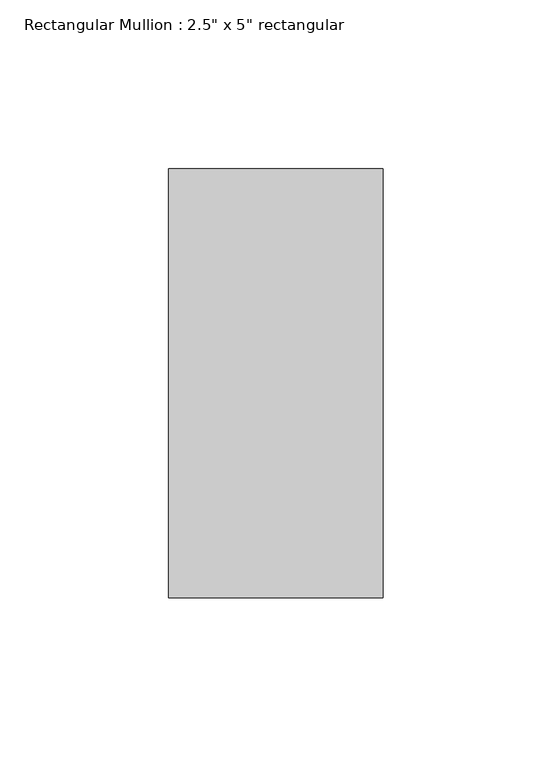
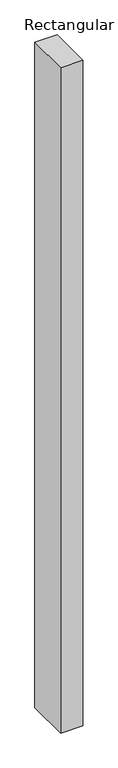
"""IFC4 building model written with IfcOpenShell, lengths in millimetres: member geometry."""

from ifc_helpers import new_model, si_unit, frame, origin, place, context, project, spatial, polyline, outline, extrude, source, transform, mapped, element, save


def member_6f41c4f0(model_context):
    return source(origin(), model_context, "Body", "SweptSolid", [
        extrude(outline(polyline([(31.75, 63.5), (31.75, -63.5), (-31.75, -63.5), (-31.75, 63.5), (31.75, 63.5)])), frame((0.0, 0.0, -2009.4971724), z_axis=(0.0, 0.0, 1.0), x_axis=(1.0, 0.0, 0.0)), (0.0, 0.0, 1.0), 2009.4971724),
    ])


if __name__ == "__main__":
    model = new_model("IFC4")
    model_context = context("Model", 3, world=origin())
    ifc_project = project(units=[si_unit("LENGTHUNIT", "METRE", prefix="MILLI")], contexts=[model_context])
    site = spatial("IfcSite", under=ifc_project)
    building = spatial("IfcBuilding", under=site)
    placement = place(None, origin())
    member_shape = member_6f41c4f0(model_context)
    element("IfcMember", 1, ObjectType="Rectangular Mullion : 2.5\" x 5\" rectangular", at=placement, inside=building, context=model_context, shape_type="MappedRepresentation", body=[
        mapped(member_shape, transform((0.0, 0.0, 0.0), x_axis=(1.0, 0.0, 0.0), y_axis=(0.0, 1.0, 0.0), z_axis=(0.0, 0.0, 1.0))),
    ])
    save(model, "model.ifc")

# Revit data of these elements
# Type "Rectangular Mullion : 2.5\" x 5\" rectangular"
#   built-in parameter 1007304 = 0.416667 (stored number, unit not read)
#   built-in parameter 1007301 = 0.104167 (stored number, unit not read)
#   built-in parameter 1007300 = 0.104167 (stored number, unit not read)
# Element 1 (IfcMember, "Rectangular Mullion : 2.5\" x 5\" rectangular")
#   Materials on its faces: "Aluminum"
# Materials
#   "Aluminum": class "Metal", colour RGB 247 247 247, transparency 0, Description = "Aluminum 6061", Cost = 0
